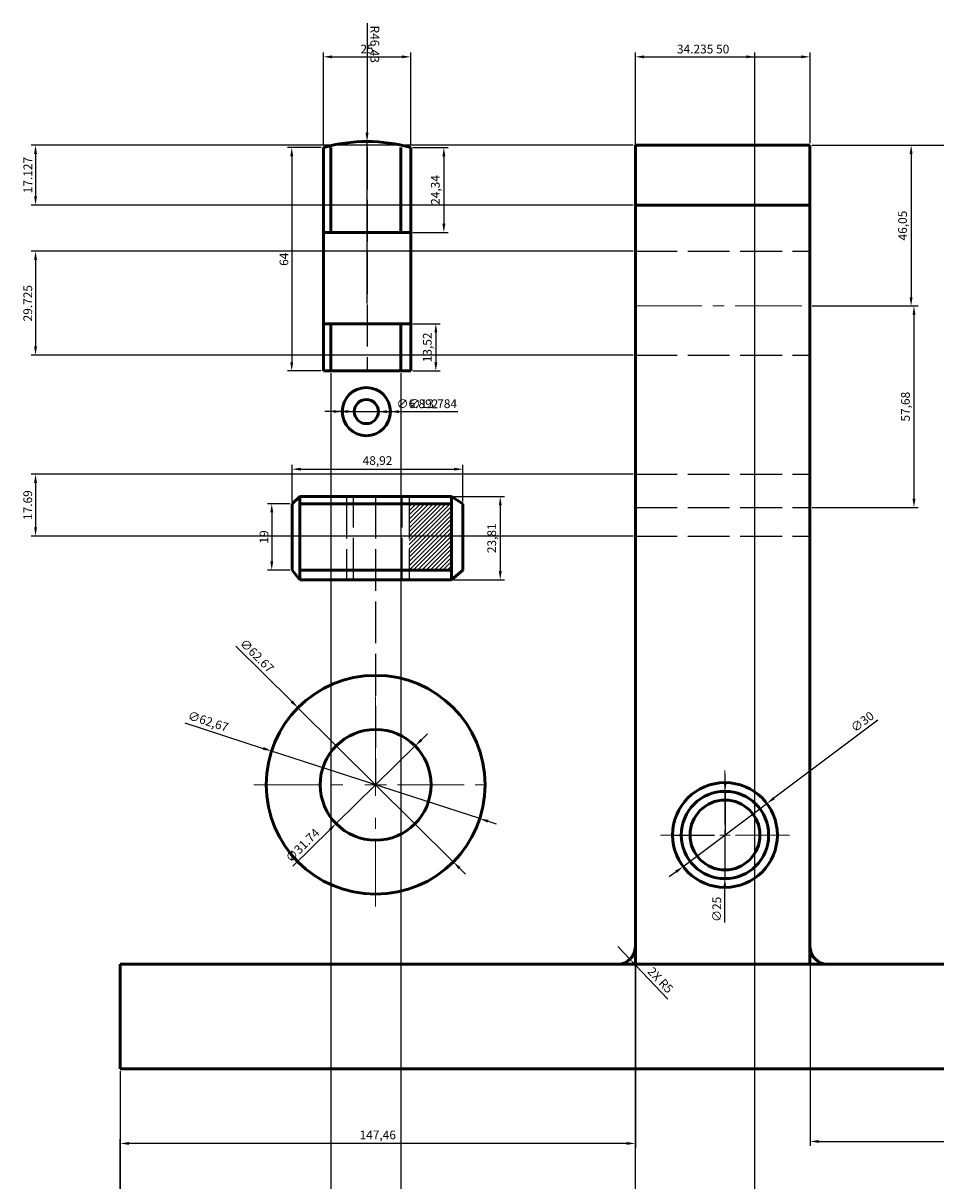
# Model space of a CAD drawing. Units: millimetres. Extents: x 921 to 2648, y 1390 to 2315.
# Tile 2 of 10: x 923 to 1184, y 1882 to 2213. Entities that reach past the tile are written whole.
import ezdxf

# ---------------------------------------------------------------- set-up
doc = ezdxf.new("R2010")
doc.units = ezdxf.units.MM
doc.linetypes.add('ACAD_ISO02W100', pattern=[15, 12, -3])
doc.linetypes.add('CENTER2', pattern=[28.575, 19.05, -3.175, 3.175, -3.175])
for name, color, linetype, lineweight in [('M-CNTR', 1, 'CENTER2', 18), ('M-DIMS', 2, 'Continuous', 25), ('M-HATC', 8, 'Continuous', 18), ('M-HIDN', 4, 'ACAD_ISO02W100', 25), ('M-OUTL', 7, 'Continuous', 50)]:
    doc.layers.add(name, color=color, linetype=linetype, lineweight=lineweight)
doc.styles.get("Standard").update_dxf_attribs({"font": 'arial.ttf'})
doc.dimstyles.new('ISO-25', dxfattribs={"dimtxt": 2.5, "dimasz": 2.5, "dimexe": 1.25, "dimexo": 0.625, "dimtad": 1, "dimtxsty": 'Standard', "dimcen": 2.5, "dimadec": 0, "dimazin": 0, "dimtfac": 1, "dimtmove": 0, "dimatfit": 3, "dimfxl": 1, "dimarcsym": 0})

# ---------------------------------------------------------------- blocks, each defined once
blk = doc.blocks.new('*D1')
at = {"layer": 'Defpoints', "color": 0, "transparency": 16777216}
for p in [(1033.77, 2177.55), (1033.77, 2153.21), (1043.26, 2153.21)]:
    blk.add_point(p, dxfattribs=at)
at = {"layer": 'M-DIMS', "color": 0, "lineweight": -2, "transparency": 16777216}
for p, q in [((1034.4, 2177.55), (1044.51, 2177.55)), ((1043.26, 2175.05), (1043.26, 2155.71)), ((1034.4, 2153.21), (1044.51, 2153.21))]:
    blk.add_line(p, q, dxfattribs=at)
at = {"layer": 'M-DIMS', "color": 0, "transparency": 16777216}
for points in [[(1042.85, 2175.05), (1043.68, 2175.05), (1043.26, 2177.55)], [(1042.85, 2155.71), (1043.68, 2155.71), (1043.26, 2153.21)]]:
    blk.add_solid(points, dxfattribs=at)
at = {"layer": 'M-DIMS', "color": 0, "transparency": 16777216, "insert": (1041.14, 2165.38), "char_height": 2.5, "attachment_point": 5, "rotation": 90}
blk.add_mtext('24,34', dxfattribs=at)
blk = doc.blocks.new('*D2')
at = {"layer": 'Defpoints', "color": 0, "transparency": 16777216}
for p in [(1033.77, 2127.07), (1033.77, 2113.55), (1040.96, 2113.55)]:
    blk.add_point(p, dxfattribs=at)
at = {"layer": 'M-DIMS', "color": 0, "lineweight": -2, "transparency": 16777216}
for p, q in [((1034.4, 2127.07), (1042.21, 2127.07)), ((1040.96, 2124.57), (1040.96, 2116.05)), ((1034.4, 2113.55), (1042.21, 2113.55))]:
    blk.add_line(p, q, dxfattribs=at)
at = {"layer": 'M-DIMS', "color": 0, "transparency": 16777216}
for points in [[(1040.55, 2124.57), (1041.38, 2124.57), (1040.96, 2127.07)], [(1040.55, 2116.05), (1041.38, 2116.05), (1040.96, 2113.55)]]:
    blk.add_solid(points, dxfattribs=at)
at = {"layer": 'M-DIMS', "color": 0, "transparency": 16777216, "insert": (1038.84, 2120.31), "char_height": 2.5, "attachment_point": 5, "rotation": 90}
blk.add_mtext('13,52', dxfattribs=at)
blk = doc.blocks.new('*D3')
at = {"layer": 'Defpoints', "color": 0, "transparency": 16777216}
for p in [(1008.77, 2177.55), (999.71, 2113.55), (1008.77, 2113.55)]:
    blk.add_point(p, dxfattribs=at)
at = {"layer": 'M-DIMS', "color": 0, "lineweight": -2, "transparency": 16777216}
for p, q in [((1008.15, 2177.55), (998.46, 2177.55)), ((999.71, 2175.05), (999.71, 2116.05)), ((1008.15, 2113.55), (998.46, 2113.55))]:
    blk.add_line(p, q, dxfattribs=at)
at = {"layer": 'M-DIMS', "color": 0, "transparency": 16777216}
for points in [[(999.29, 2175.05), (1000.12, 2175.05), (999.71, 2177.55)], [(999.29, 2116.05), (1000.12, 2116.05), (999.71, 2113.55)]]:
    blk.add_solid(points, dxfattribs=at)
at = {"layer": 'M-DIMS', "color": 0, "transparency": 16777216, "insert": (997.8, 2145.55), "char_height": 2.5, "attachment_point": 5, "rotation": 90}
blk.add_mtext('64', dxfattribs=at)
blk = doc.blocks.new('*U4')
at = {"layer": 'M-CNTR', "color": 0, "transparency": 16777216}
for p, q in [((0, 6.27), (0, 34.83)), ((-34.83, 0), (-6.27, 0)), ((6.27, 0), (34.83, 0)), ((0, -34.83), (0, -6.27))]:
    blk.add_line(p, q, dxfattribs=at)
at = {"layer": 'M-CNTR', "color": 0, "linetype": 'Continuous', "transparency": 16777216}
for p, q in [((-3.13, 0), (3.13, 0)), ((0, -3.13), (0, 3.13))]:
    blk.add_line(p, q, dxfattribs=at)
blk = doc.blocks.new('*U5')
at = {"layer": 'M-CNTR', "color": 0, "transparency": 16777216}
for p, q in [((0, 3), (0, 18.5)), ((-18.5, 0), (-3, 0)), ((3, 0), (18.5, 0)), ((0, -18.5), (0, -3))]:
    blk.add_line(p, q, dxfattribs=at)
at = {"layer": 'M-CNTR', "color": 0, "linetype": 'Continuous', "transparency": 16777216}
for p, q in [((-1.5, 0), (1.5, 0)), ((0, -1.5), (0, 1.5))]:
    blk.add_line(p, q, dxfattribs=at)
blk = doc.blocks.new('*D6')
at = {"layer": 'Defpoints', "color": 0, "transparency": 16777216}
for p in [(1048.72, 2085.43), (999.8, 2075.52), (1048.72, 2075.52)]:
    blk.add_point(p, dxfattribs=at)
at = {"layer": 'M-DIMS', "color": 0, "lineweight": -2, "transparency": 16777216}
for p, q in [((999.8, 2076.14), (999.8, 2086.68)), ((1002.3, 2085.43), (1046.22, 2085.43)), ((1048.72, 2076.14), (1048.72, 2086.68))]:
    blk.add_line(p, q, dxfattribs=at)
at = {"layer": 'M-DIMS', "color": 0, "transparency": 16777216}
for points in [[(1002.3, 2085.85), (1002.3, 2085.01), (999.8, 2085.43)], [(1046.22, 2085.85), (1046.22, 2085.01), (1048.72, 2085.43)]]:
    blk.add_solid(points, dxfattribs=at)
at = {"layer": 'M-DIMS', "color": 0, "transparency": 16777216, "insert": (1024.26, 2087.56), "char_height": 2.5, "attachment_point": 5}
blk.add_mtext('48,92', dxfattribs=at)
blk = doc.blocks.new('*D7')
at = {"layer": 'Defpoints', "color": 0, "transparency": 16777216}
for p in [(1045.45, 2077.56), (1045.45, 2053.75), (1059.4, 2053.75)]:
    blk.add_point(p, dxfattribs=at)
at = {"layer": 'M-DIMS', "color": 0, "lineweight": -2, "transparency": 16777216}
for p, q in [((1046.07, 2077.56), (1060.65, 2077.56)), ((1059.4, 2075.06), (1059.4, 2056.25)), ((1046.07, 2053.75), (1060.65, 2053.75))]:
    blk.add_line(p, q, dxfattribs=at)
at = {"layer": 'M-DIMS', "color": 0, "transparency": 16777216}
for points in [[(1058.99, 2075.06), (1059.82, 2075.06), (1059.4, 2077.56)], [(1058.99, 2056.25), (1059.82, 2056.25), (1059.4, 2053.75)]]:
    blk.add_solid(points, dxfattribs=at)
at = {"layer": 'M-DIMS', "color": 0, "transparency": 16777216, "insert": (1057.28, 2065.65), "char_height": 2.5, "attachment_point": 5, "rotation": 90}
blk.add_mtext('23,81', dxfattribs=at)
blk = doc.blocks.new('*D8')
at = {"layer": 'Defpoints', "color": 0, "transparency": 16777216}
for p in [(999.8, 2075.52), (993.99, 2056.52), (999.8, 2056.52)]:
    blk.add_point(p, dxfattribs=at)
at = {"layer": 'M-DIMS', "color": 0, "lineweight": -2, "transparency": 16777216}
for p, q in [((999.18, 2075.52), (992.74, 2075.52)), ((993.99, 2073.02), (993.99, 2059.02)), ((999.18, 2056.52), (992.74, 2056.52))]:
    blk.add_line(p, q, dxfattribs=at)
at = {"layer": 'M-DIMS', "color": 0, "transparency": 16777216}
for points in [[(993.57, 2073.02), (994.41, 2073.02), (993.99, 2075.52)], [(993.57, 2059.02), (994.41, 2059.02), (993.99, 2056.52)]]:
    blk.add_solid(points, dxfattribs=at)
at = {"layer": 'M-DIMS', "color": 0, "transparency": 16777216, "insert": (992.09, 2066.02), "char_height": 2.5, "attachment_point": 5, "rotation": 90}
blk.add_mtext('19', dxfattribs=at)
blk = doc.blocks.new('*D9')
at = {"layer": 'Defpoints', "color": 0, "transparency": 16777216}
for p in [(993.92, 2004.7), (1053.53, 1985.37)]:
    blk.add_point(p, dxfattribs=at)
at = {"layer": 'M-DIMS', "color": 0, "lineweight": -2, "transparency": 16777216}
for p, q in [((969.13, 2012.74), (991.54, 2005.47)), ((1053.53, 1985.37), (993.92, 2004.7)), ((1055.91, 1984.6), (1058.28, 1983.83))]:
    blk.add_line(p, q, dxfattribs=at)
at = {"layer": 'M-DIMS', "color": 0, "transparency": 16777216}
for points in [[(991.67, 2005.87), (991.41, 2005.08), (993.92, 2004.7)], [(1056.03, 1984.99), (1055.78, 1984.2), (1053.53, 1985.37)]]:
    blk.add_solid(points, dxfattribs=at)
at = {"layer": 'M-DIMS', "color": 0, "transparency": 16777216, "insert": (975.7, 2012.89), "char_height": 2.5, "attachment_point": 5, "rotation": 342.0306}
blk.add_mtext('∅62,67', dxfattribs=at)
blk = doc.blocks.new('*D10')
at = {"layer": 'Defpoints', "color": 0, "transparency": 16777216}
for p in [(1148.08, 2178.21), (1148.08, 2132.16), (1177.03, 2132.16)]:
    blk.add_point(p, dxfattribs=at)
at = {"layer": 'M-DIMS', "color": 0, "lineweight": -2, "transparency": 16777216}
for p, q in [((1148.7, 2178.21), (1178.28, 2178.21)), ((1177.03, 2175.71), (1177.03, 2134.66)), ((1148.7, 2132.16), (1178.28, 2132.16))]:
    blk.add_line(p, q, dxfattribs=at)
at = {"layer": 'M-DIMS', "color": 0, "transparency": 16777216}
for points in [[(1176.61, 2175.71), (1177.44, 2175.71), (1177.03, 2178.21)], [(1176.61, 2134.66), (1177.44, 2134.66), (1177.03, 2132.16)]]:
    blk.add_solid(points, dxfattribs=at)
at = {"layer": 'M-DIMS', "color": 0, "transparency": 16777216, "insert": (1174.9, 2155.19), "char_height": 2.5, "attachment_point": 5, "rotation": 90}
blk.add_mtext('46,05', dxfattribs=at)
blk = doc.blocks.new('*D11')
at = {"layer": 'Defpoints', "color": 0, "transparency": 16777216}
for p in [(1148.08, 2132.16), (1148.08, 2074.48), (1177.84, 2074.48)]:
    blk.add_point(p, dxfattribs=at)
at = {"layer": 'M-DIMS', "color": 0, "lineweight": -2, "transparency": 16777216}
for p, q in [((1148.7, 2132.16), (1179.09, 2132.16)), ((1177.84, 2129.66), (1177.84, 2076.98)), ((1148.7, 2074.48), (1179.09, 2074.48))]:
    blk.add_line(p, q, dxfattribs=at)
at = {"layer": 'M-DIMS', "color": 0, "transparency": 16777216}
for points in [[(1177.43, 2129.66), (1178.26, 2129.66), (1177.84, 2132.16)], [(1177.43, 2076.98), (1178.26, 2076.98), (1177.84, 2074.48)]]:
    blk.add_solid(points, dxfattribs=at)
at = {"layer": 'M-DIMS', "color": 0, "transparency": 16777216, "insert": (1175.72, 2103.32), "char_height": 2.5, "attachment_point": 5, "rotation": 90}
blk.add_mtext('57,68', dxfattribs=at)
blk = doc.blocks.new('*D12')
at = {"layer": 'Defpoints', "color": 0, "transparency": 16777216}
for p in [(1135.73, 1989.67), (1111.75, 1971.64)]:
    blk.add_point(p, dxfattribs=at)
at = {"layer": 'M-DIMS', "color": 0, "lineweight": -2, "transparency": 16777216}
for p, q in [((1167.46, 2013.52), (1137.73, 1991.17)), ((1111.75, 1971.64), (1135.73, 1989.67)), ((1109.75, 1970.14), (1107.75, 1968.64))]:
    blk.add_line(p, q, dxfattribs=at)
at = {"layer": 'M-DIMS', "color": 0, "transparency": 16777216}
for points in [[(1137.48, 1991.5), (1137.98, 1990.84), (1135.73, 1989.67)], [(1109.5, 1970.47), (1110, 1969.81), (1111.75, 1971.64)]]:
    blk.add_solid(points, dxfattribs=at)
at = {"layer": 'M-DIMS', "color": 0, "transparency": 16777216, "insert": (1163.26, 2012.83), "char_height": 2.5, "attachment_point": 5, "rotation": 36.9285}
blk.add_mtext('∅30', dxfattribs=at)
blk = doc.blocks.new('*D17')
at = {"layer": 'Defpoints', "color": 0, "transparency": 16777216}
for p in [(1098.08, 1948.7), (950.61, 1892.33), (950.61, 1878.16)]:
    blk.add_point(p, dxfattribs=at)
at = {"layer": 'M-DIMS', "color": 0, "lineweight": -2, "transparency": 16777216}
for p, q in [((1098.08, 1948.07), (1098.08, 1891.08)), ((950.61, 1878.78), (950.61, 1893.58)), ((1095.58, 1892.33), (953.11, 1892.33))]:
    blk.add_line(p, q, dxfattribs=at)
at = {"layer": 'M-DIMS', "color": 0, "transparency": 16777216}
for points in [[(953.11, 1892.74), (953.11, 1891.91), (950.61, 1892.33)], [(1095.58, 1892.74), (1095.58, 1891.91), (1098.08, 1892.33)]]:
    blk.add_solid(points, dxfattribs=at)
at = {"layer": 'M-DIMS', "color": 0, "transparency": 16777216, "insert": (1024.34, 1894.45), "char_height": 2.5, "attachment_point": 5}
blk.add_mtext('147,46', dxfattribs=at)
blk = doc.blocks.new('*D18')
at = {"layer": 'Defpoints', "color": 0, "transparency": 16777216}
for p in [(1148.08, 1948.7), (1294.79, 1892.9), (1294.79, 1878.16)]:
    blk.add_point(p, dxfattribs=at)
at = {"layer": 'M-DIMS', "color": 0, "lineweight": -2, "transparency": 16777216}
for p, q in [((1148.08, 1948.07), (1148.08, 1891.65)), ((1294.79, 1878.78), (1294.79, 1894.15)), ((1150.58, 1892.9), (1292.29, 1892.9))]:
    blk.add_line(p, q, dxfattribs=at)
at = {"layer": 'M-DIMS', "color": 0, "transparency": 16777216}
for points in [[(1150.58, 1893.32), (1150.58, 1892.48), (1148.08, 1892.9)], [(1292.29, 1893.32), (1292.29, 1892.48), (1294.79, 1892.9)]]:
    blk.add_solid(points, dxfattribs=at)
at = {"layer": 'M-DIMS', "color": 0, "transparency": 16777216, "insert": (1221.43, 1895.03), "char_height": 2.5, "attachment_point": 5}
blk.add_mtext('146,72', dxfattribs=at)
blk = doc.blocks.new('*D41')
at = {"layer": 'Defpoints', "color": 0, "transparency": 16777216}
for p in [(1148.08, 2203.51), (1098.08, 2178.21), (1148.08, 2178.21)]:
    blk.add_point(p, dxfattribs=at)
at = {"layer": 'M-DIMS', "color": 0, "lineweight": -2, "transparency": 16777216}
for p, q in [((1098.08, 2178.83), (1098.08, 2204.76)), ((1100.58, 2203.51), (1145.58, 2203.51)), ((1148.08, 2178.83), (1148.08, 2204.76))]:
    blk.add_line(p, q, dxfattribs=at)
at = {"layer": 'M-DIMS', "color": 0, "transparency": 16777216}
for points in [[(1100.58, 2203.93), (1100.58, 2203.1), (1098.08, 2203.51)], [(1145.58, 2203.93), (1145.58, 2203.1), (1148.08, 2203.51)]]:
    blk.add_solid(points, dxfattribs=at)
at = {"layer": 'M-DIMS', "color": 0, "transparency": 16777216, "insert": (1123.08, 2205.42), "char_height": 2.5, "attachment_point": 5}
blk.add_mtext('50', dxfattribs=at)
blk = doc.blocks.new('*D42')
at = {"layer": 'Defpoints', "color": 0, "transparency": 16777216}
for p in [(1098.08, 2178.21), (926.36, 2161.08), (1098.08, 2161.08)]:
    blk.add_point(p, dxfattribs=at)
at = {"layer": 'M-DIMS', "color": 0, "lineweight": -2, "transparency": 16777216}
for p, q in [((1097.45, 2178.21), (925.11, 2178.21)), ((926.36, 2175.71), (926.36, 2163.58)), ((1097.45, 2161.08), (925.11, 2161.08))]:
    blk.add_line(p, q, dxfattribs=at)
at = {"layer": 'M-DIMS', "color": 0, "transparency": 16777216}
for points in [[(925.95, 2175.71), (926.78, 2175.71), (926.36, 2178.21)], [(925.95, 2163.58), (926.78, 2163.58), (926.36, 2161.08)]]:
    blk.add_solid(points, dxfattribs=at)
at = {"layer": 'M-DIMS', "color": 0, "transparency": 16777216, "insert": (924.48, 2169.65), "char_height": 2.5, "attachment_point": 5, "rotation": 90}
blk.add_mtext('17.127', dxfattribs=at)
blk = doc.blocks.new('*D43')
at = {"layer": 'Defpoints', "color": 0, "transparency": 16777216}
for p in [(1098.08, 2147.83), (926.36, 2118.1), (1098.08, 2118.1)]:
    blk.add_point(p, dxfattribs=at)
at = {"layer": 'M-DIMS', "color": 0, "lineweight": -2, "transparency": 16777216}
for p, q in [((1097.45, 2147.83), (925.11, 2147.83)), ((926.36, 2145.33), (926.36, 2120.6)), ((1097.45, 2118.1), (925.11, 2118.1))]:
    blk.add_line(p, q, dxfattribs=at)
at = {"layer": 'M-DIMS', "color": 0, "transparency": 16777216}
for points in [[(925.95, 2145.33), (926.78, 2145.33), (926.36, 2147.83)], [(925.95, 2120.6), (926.78, 2120.6), (926.36, 2118.1)]]:
    blk.add_solid(points, dxfattribs=at)
at = {"layer": 'M-DIMS', "color": 0, "transparency": 16777216, "insert": (924.46, 2132.96), "char_height": 2.5, "attachment_point": 5, "rotation": 90}
blk.add_mtext('29.725', dxfattribs=at)
blk = doc.blocks.new('*D44')
at = {"layer": 'Defpoints', "color": 0, "transparency": 16777216}
for p in [(1098.08, 2083.98), (926.36, 2066.28), (1098.08, 2066.28)]:
    blk.add_point(p, dxfattribs=at)
at = {"layer": 'M-DIMS', "color": 0, "lineweight": -2, "transparency": 16777216}
for p, q in [((1097.45, 2083.98), (925.11, 2083.98)), ((926.36, 2081.48), (926.36, 2068.78)), ((1097.45, 2066.28), (925.11, 2066.28))]:
    blk.add_line(p, q, dxfattribs=at)
at = {"layer": 'M-DIMS', "color": 0, "transparency": 16777216}
for points in [[(925.95, 2081.48), (926.78, 2081.48), (926.36, 2083.98)], [(925.95, 2068.78), (926.78, 2068.78), (926.36, 2066.28)]]:
    blk.add_solid(points, dxfattribs=at)
at = {"layer": 'M-DIMS', "color": 0, "transparency": 16777216, "insert": (924.46, 2075.13), "char_height": 2.5, "attachment_point": 5, "rotation": 90}
blk.add_mtext('17.69', dxfattribs=at)
blk = doc.blocks.new('*D46')
at = {"layer": 'Defpoints', "color": 0, "transparency": 16777216}
for p in [(1148.08, 2178.21), (1294.79, 1913.7), (1319.04, 1913.7)]:
    blk.add_point(p, dxfattribs=at)
at = {"layer": 'M-DIMS', "color": 0, "lineweight": -2, "transparency": 16777216}
for p, q in [((1148.7, 2178.21), (1320.29, 2178.21)), ((1319.04, 2175.71), (1319.04, 1916.2)), ((1295.42, 1913.7), (1320.29, 1913.7))]:
    blk.add_line(p, q, dxfattribs=at)
at = {"layer": 'M-DIMS', "color": 0, "transparency": 16777216}
for points in [[(1318.63, 2175.71), (1319.46, 2175.71), (1319.04, 2178.21)], [(1318.63, 1916.2), (1319.46, 1916.2), (1319.04, 1913.7)]]:
    blk.add_solid(points, dxfattribs=at)
at = {"layer": 'M-DIMS', "color": 0, "transparency": 16777216, "insert": (1317.14, 2045.95), "char_height": 2.5, "attachment_point": 5, "rotation": 90}
blk.add_mtext('264.5', dxfattribs=at)
blk = doc.blocks.new('*D49')
at = {"layer": 'Defpoints', "color": 0, "transparency": 16777216}
for p in [(950.61, 1913.7), (1294.79, 1913.7), (1294.79, 1705.98)]:
    blk.add_point(p, dxfattribs=at)
at = {"layer": 'M-DIMS', "color": 0, "lineweight": -2, "transparency": 16777216}
for p, q in [((950.61, 1913.07), (950.61, 1704.73)), ((1294.79, 1913.07), (1294.79, 1704.73)), ((953.11, 1705.98), (1292.29, 1705.98))]:
    blk.add_line(p, q, dxfattribs=at)
at = {"layer": 'M-DIMS', "color": 0, "transparency": 16777216}
for points in [[(953.11, 1706.4), (953.11, 1705.56), (950.61, 1705.98)], [(1292.29, 1706.4), (1292.29, 1705.56), (1294.79, 1705.98)]]:
    blk.add_solid(points, dxfattribs=at)
at = {"layer": 'M-DIMS', "color": 0, "transparency": 16777216, "insert": (1122.7, 1707.88), "char_height": 2.5, "attachment_point": 5}
blk.add_mtext('344.2', dxfattribs=at)
blk = doc.blocks.new('*D51')
at = {"layer": 'Defpoints', "color": 0, "transparency": 16777216}
for p in [(1132.31, 2203.51), (1098.08, 1817.38), (1132.31, 1818.84)]:
    blk.add_point(p, dxfattribs=at)
at = {"layer": 'M-DIMS', "color": 0, "lineweight": -2, "transparency": 16777216}
for p, q in [((1098.08, 1818), (1098.08, 2204.76)), ((1100.58, 2203.51), (1129.81, 2203.51)), ((1132.31, 1819.47), (1132.31, 2204.76))]:
    blk.add_line(p, q, dxfattribs=at)
at = {"layer": 'M-DIMS', "color": 0, "transparency": 16777216}
for points in [[(1100.58, 2203.93), (1100.58, 2203.1), (1098.08, 2203.51)], [(1129.81, 2203.93), (1129.81, 2203.1), (1132.31, 2203.51)]]:
    blk.add_solid(points, dxfattribs=at)
at = {"layer": 'M-DIMS', "color": 0, "transparency": 16777216, "insert": (1115.19, 2205.42), "char_height": 2.5, "attachment_point": 5}
blk.add_mtext('34.235', dxfattribs=at)
blk = doc.blocks.new('*D52')
at = {"layer": 'Defpoints', "color": 0, "transparency": 16777216}
for p in [(1033.77, 2203.51), (1008.77, 2177.55), (1033.77, 2177.55)]:
    blk.add_point(p, dxfattribs=at)
at = {"layer": 'M-DIMS', "color": 0, "lineweight": -2, "transparency": 16777216}
for p, q in [((1008.77, 2178.18), (1008.77, 2204.76)), ((1011.27, 2203.51), (1031.27, 2203.51)), ((1033.77, 2178.18), (1033.77, 2204.76))]:
    blk.add_line(p, q, dxfattribs=at)
at = {"layer": 'M-DIMS', "color": 0, "transparency": 16777216}
for points in [[(1011.27, 2203.93), (1011.27, 2203.1), (1008.77, 2203.51)], [(1031.27, 2203.93), (1031.27, 2203.1), (1033.77, 2203.51)]]:
    blk.add_solid(points, dxfattribs=at)
at = {"layer": 'M-DIMS', "color": 0, "transparency": 16777216, "insert": (1021.27, 2205.42), "char_height": 2.5, "attachment_point": 5}
blk.add_mtext('25', dxfattribs=at)
blk = doc.blocks.new('*D53')
at = {"layer": 'Defpoints', "color": 0, "transparency": 16777216}
for p in [(1010.93, 2113.55), (1030.91, 2113.55), (1030.91, 1705.98)]:
    blk.add_point(p, dxfattribs=at)
at = {"layer": 'M-DIMS', "color": 0, "lineweight": -2, "transparency": 16777216}
for p, q in [((1010.93, 2112.93), (1010.93, 1704.73)), ((1030.91, 2112.93), (1030.91, 1704.73)), ((1013.43, 1705.98), (1028.41, 1705.98))]:
    blk.add_line(p, q, dxfattribs=at)
at = {"layer": 'M-DIMS', "color": 0, "transparency": 16777216}
for points in [[(1013.43, 1706.4), (1013.43, 1705.56), (1010.93, 1705.98)], [(1028.41, 1706.4), (1028.41, 1705.56), (1030.91, 1705.98)]]:
    blk.add_solid(points, dxfattribs=at)
at = {"layer": 'M-DIMS', "color": 0, "transparency": 16777216, "insert": (1020.92, 1707.88), "char_height": 2.5, "attachment_point": 5}
blk.add_mtext('19.983', dxfattribs=at)
blk = doc.blocks.new('*D121')
at = {"layer": 'Defpoints', "color": 0, "transparency": 16777216}
for p in [(1021.27, 2179.26), (1021.27, 2132.84)]:
    blk.add_point(p, dxfattribs=at)
at = {"layer": 'M-DIMS', "color": 0, "lineweight": -2, "transparency": 16777216}
for p, q in [((1021.27, 2213.16), (1021.27, 2181.76)), ((1021.27, 2132.84), (1021.27, 2179.26))]:
    blk.add_line(p, q, dxfattribs=at)
at = {"layer": 'M-DIMS', "color": 0, "transparency": 16777216}
blk.add_solid([(1021.69, 2181.76), (1020.85, 2181.76), (1021.27, 2179.26)], dxfattribs=at)
at = {"layer": 'M-DIMS', "color": 0, "transparency": 16777216, "insert": (1023.17, 2207.12), "char_height": 2.5, "attachment_point": 5, "rotation": 270.0002}
blk.add_mtext('R46.43', dxfattribs=at)
blk = doc.blocks.new('*D123')
at = {"layer": 'Defpoints', "color": 0, "transparency": 16777216}
for p in [(1001.49, 2017.11), (1045.96, 1972.96)]:
    blk.add_point(p, dxfattribs=at)
at = {"layer": 'M-DIMS', "color": 0, "lineweight": -2, "transparency": 16777216}
for p, q in [((983.75, 2034.73), (999.71, 2018.87)), ((1045.96, 1972.96), (1001.49, 2017.11)), ((1047.73, 1971.19), (1049.5, 1969.43))]:
    blk.add_line(p, q, dxfattribs=at)
at = {"layer": 'M-DIMS', "color": 0, "transparency": 16777216}
for points in [[(1000.01, 2019.17), (999.42, 2018.58), (1001.49, 2017.11)], [(1048.02, 1971.49), (1047.44, 1970.9), (1045.96, 1972.96)]]:
    blk.add_solid(points, dxfattribs=at)
at = {"layer": 'M-DIMS', "color": 0, "transparency": 16777216, "insert": (989.54, 2031.76), "char_height": 2.5, "attachment_point": 5, "rotation": 315.2017}
blk.add_mtext('∅62.67', dxfattribs=at)
blk = doc.blocks.new('*D124')
at = {"layer": 'Defpoints', "color": 0, "transparency": 16777216}
for p in [(1035.04, 2006.16), (1012.41, 1983.91)]:
    blk.add_point(p, dxfattribs=at)
at = {"layer": 'M-DIMS', "color": 0, "lineweight": -2, "transparency": 16777216}
for p, q in [((1036.82, 2007.91), (1038.6, 2009.67)), ((1035.04, 2006.16), (1012.41, 1983.91)), ((1000.01, 1971.71), (1010.63, 1982.15))]:
    blk.add_line(p, q, dxfattribs=at)
at = {"layer": 'M-DIMS', "color": 0, "transparency": 16777216}
for points in [[(1036.53, 2008.21), (1037.11, 2007.62), (1035.04, 2006.16)], [(1010.33, 1982.45), (1010.92, 1981.86), (1012.41, 1983.91)]]:
    blk.add_solid(points, dxfattribs=at)
at = {"layer": 'M-DIMS', "color": 0, "transparency": 16777216, "insert": (1003.04, 1977.46), "char_height": 2.5, "attachment_point": 5, "rotation": 44.525}
blk.add_mtext('∅31.74', dxfattribs=at)
blk = doc.blocks.new('*D126')
at = {"layer": 'Defpoints', "color": 0, "transparency": 16777216}
for p in [(1093.08, 1948.7), (1096.52, 1945.07)]:
    blk.add_point(p, dxfattribs=at)
at = {"layer": 'M-DIMS', "color": 0, "lineweight": -2, "transparency": 16777216}
for p, q in [((1093.08, 1948.7), (1096.52, 1945.07)), ((1107.34, 1933.68), (1098.24, 1943.26))]:
    blk.add_line(p, q, dxfattribs=at)
at = {"layer": 'M-DIMS', "color": 0, "transparency": 16777216}
blk.add_solid([(1098.54, 1943.55), (1097.94, 1942.97), (1096.52, 1945.07)], dxfattribs=at)
at = {"layer": 'M-DIMS', "color": 0, "transparency": 16777216, "insert": (1105.03, 1938.88), "char_height": 2.5, "attachment_point": 5, "rotation": 313.5346}
blk.add_mtext('2X R5', dxfattribs=at)
blk = doc.blocks.new('*D127')
at = {"layer": 'Defpoints', "color": 0, "transparency": 16777216}
for p in [(1123.78, 1993.16), (1123.7, 1968.16)]:
    blk.add_point(p, dxfattribs=at)
at = {"layer": 'M-DIMS', "color": 0, "lineweight": -2, "transparency": 16777216}
for p, q in [((1123.79, 1995.66), (1123.8, 1998.16)), ((1123.78, 1993.16), (1123.7, 1968.16)), ((1123.66, 1955.59), (1123.69, 1965.66))]:
    blk.add_line(p, q, dxfattribs=at)
at = {"layer": 'M-DIMS', "color": 0, "transparency": 16777216}
for points in [[(1123.37, 1995.66), (1124.21, 1995.65), (1123.78, 1993.16)], [(1123.28, 1965.66), (1124.11, 1965.65), (1123.7, 1968.16)]]:
    blk.add_solid(points, dxfattribs=at)
at = {"layer": 'M-DIMS', "color": 0, "transparency": 16777216, "insert": (1121.7, 1959.38), "char_height": 2.5, "attachment_point": 5, "rotation": 89.8137}
blk.add_mtext('∅25', dxfattribs=at)
blk = doc.blocks.new('*D128')
at = {"layer": 'Defpoints', "color": 0, "transparency": 16777216}
for p in [(1014.17, 2101.93), (1027.95, 2101.9)]:
    blk.add_point(p, dxfattribs=at)
at = {"layer": 'M-DIMS', "color": 0, "lineweight": -2, "transparency": 16777216}
for p, q in [((1011.67, 2101.93), (1009.17, 2101.94)), ((1014.17, 2101.93), (1027.95, 2101.9)), ((1047.29, 2101.86), (1030.45, 2101.89))]:
    blk.add_line(p, q, dxfattribs=at)
at = {"layer": 'M-DIMS', "color": 0, "transparency": 16777216}
for points in [[(1011.67, 2102.35), (1011.67, 2101.52), (1014.17, 2101.93)], [(1030.45, 2102.31), (1030.45, 2101.48), (1027.95, 2101.9)]]:
    blk.add_solid(points, dxfattribs=at)
at = {"layer": 'M-DIMS', "color": 0, "transparency": 16777216, "insert": (1040.12, 2103.85), "char_height": 2.5, "attachment_point": 5, "rotation": 359.8848}
blk.add_mtext('∅13.784', dxfattribs=at)
blk = doc.blocks.new('*D129')
at = {"layer": 'Defpoints', "color": 0, "transparency": 16777216}
for p in [(1017.61, 2101.93), (1024.51, 2101.9)]:
    blk.add_point(p, dxfattribs=at)
at = {"layer": 'M-DIMS', "color": 0, "lineweight": -2, "transparency": 16777216}
for p, q in [((1015.11, 2101.94), (1012.61, 2101.95)), ((1017.61, 2101.93), (1024.51, 2101.9)), ((1041.89, 2101.83), (1027.01, 2101.89))]:
    blk.add_line(p, q, dxfattribs=at)
at = {"layer": 'M-DIMS', "color": 0, "transparency": 16777216}
for points in [[(1015.12, 2102.35), (1015.11, 2101.52), (1017.61, 2101.93)], [(1027.01, 2102.31), (1027, 2101.47), (1024.51, 2101.9)]]:
    blk.add_solid(points, dxfattribs=at)
at = {"layer": 'M-DIMS', "color": 0, "transparency": 16777216, "insert": (1035.7, 2103.83), "char_height": 2.5, "attachment_point": 5, "rotation": 359.7775}
blk.add_mtext('∅6.892', dxfattribs=at)

msp = doc.modelspace()

# ---------------------------------------------------------------- hatches: boundary and pattern name
at = {"layer": 'M-HATC'}
h = msp.add_hatch(dxfattribs=at)
h.set_pattern_fill('ANSI31', color=256, scale=0.27)
h.paths.add_polyline_path([(1045.4452, 2075.5156), (1033.3358, 2075.5156), (1033.3358, 2056.5156), (1045.4452, 2056.5156)])

# ---------------------------------------------------------------- linework, layer by layer
at = {"layer": 'M-CNTR'}
msp.add_line((1098.0755, 2132.1608), (1148.0755, 2132.1608), dxfattribs=at)
at = {"layer": 'M-HIDN'}
for p, q in [((1021.2702, 2177.5505), (1021.2702, 2113.5505)), ((1098.0755, 2147.8264), (1148.0755, 2147.8264)), ((1098.0755, 2118.1019), (1148.0755, 2118.1019)), ((1098.0755, 2083.9757), (1148.0755, 2083.9757)), ((1015.4234, 2077.5571), (1015.4234, 2053.7481)), ((1017.4234, 2053.7481), (1017.4234, 2077.5571)), ((1023.7222, 2077.5571), (1023.7222, 1995.0344)), ((1031.3358, 2053.7481), (1031.3358, 2077.5571)), ((1033.3358, 2077.5571), (1033.3358, 2053.7481)), ((1098.0755, 2074.4762), (1148.0755, 2074.4762)), ((1098.0755, 2066.2842), (1148.0755, 2066.2842)), ((1108.7408, 1980.6559), (1123.7408, 1980.6559))]:
    msp.add_line(p, q, dxfattribs=at)
at = {"layer": 'M-OUTL'}
for p, q in [((1008.7702, 2177.5505), (1008.7702, 2113.5505)), ((1010.9275, 2177.5505), (1010.9275, 2153.2139)), ((1030.91, 2153.2139), (1030.91, 2177.5505)), ((1033.7702, 2113.5505), (1033.7702, 2177.5505)), ((1098.0755, 2178.2093), (1098.0755, 1948.699)), ((1098.0755, 2178.2093), (1148.0755, 2178.2093)), ((1148.0755, 1948.699), (1148.0755, 2178.2093)), ((1098.0755, 2161.082), (1148.0755, 2161.082)), ((1008.7702, 2153.2139), (1033.7702, 2153.2139)), ((1008.7702, 2127.0726), (1033.7702, 2127.0726)), ((1010.9275, 2127.0726), (1010.9275, 2113.5505)), ((1030.91, 2113.5505), (1030.91, 2127.0726)), ((1008.7702, 2113.5505), (1033.7702, 2113.5505)), ((999.8032, 2075.5156), (1001.9992, 2077.5571)), ((999.8032, 2075.5156), (999.8032, 2056.5156)), ((1001.9992, 2077.5571), (1045.4452, 2077.5571)), ((1001.9992, 2077.5571), (1001.9992, 2053.7481)), ((1001.9992, 2075.5156), (1045.4452, 2075.5156)), ((1045.4452, 2077.5571), (1045.4452, 2053.7481)), ((1045.4452, 2077.5571), (1048.7232, 2075.5156)), ((1048.7232, 2075.5156), (1048.7232, 2056.5156)), ((999.8032, 2056.5156), (1001.9992, 2053.7481)), ((1045.4452, 2056.5156), (1001.9992, 2056.5156)), ((1045.4452, 2053.7481), (1048.7232, 2056.5156)), ((1045.4452, 2053.7481), (1001.9992, 2053.7481)), ((1098.0755, 1948.699), (1098.0755, 1943.699)), ((1148.0755, 1948.699), (1148.0755, 1943.699)), ((1093.0755, 1943.699), (950.6135, 1943.699)), ((950.6135, 1943.699), (950.6135, 1913.699)), ((1098.0755, 1943.699), (1093.0755, 1943.699)), ((1098.0755, 1943.699), (1148.0755, 1943.699)), ((1148.0755, 1943.699), (1153.0755, 1943.699)), ((1294.7941, 1943.699), (1153.0755, 1943.699)), ((950.6135, 1913.699), (1294.7941, 1913.699))]:
    msp.add_line(p, q, dxfattribs=at)
for centre, radius in [((1021.0594, 2101.9138), 6.892), ((1021.0594, 2101.9138), 3.446), ((1023.7222, 1995.0344), 31.3337), ((1023.7222, 1995.0344), 15.8685), ((1123.7408, 1980.6559), 15), ((1123.7408, 1980.6559), 12.5), ((1123.7408, 1980.6559), 10)]:
    msp.add_circle(centre, radius, dxfattribs=at)
for centre, radius, start, end in [((1021.2702, 2132.8382), 46.4267, 74.38087, 105.61913), ((1093.0755, 1948.699), 5, 270, 0), ((1153.0755, 1948.699), 5, 180, 270)]:
    msp.add_arc(centre, radius, start, end, dxfattribs=at)

# ---------------------------------------------------------------- block references
at = {"layer": 'M-CNTR'}
for name, p in [('*U4', (1023.7222, 1995.0344)), ('*U5', (1123.7408, 1980.6559))]:
    msp.add_blockref(name, p, dxfattribs=at)

# ---------------------------------------------------------------- dimensions: what is measured, and where the dimension line sits
at = {"layer": 'M-DIMS'}
dim = msp.add_radius_dim(center=(1021.2702, 2132.8382), mpoint=(1021.27, 2179.2649), dimstyle='ISO-25', override={"dimdec": 2, "dimlfac": 1, "dimrnd": 0, "dimzin": 0, "dimdsep": 46, "dimlunit": 2}, dxfattribs=at)
dim.commit()
dim.dimension.update_dxf_attribs({"geometry": '*D121', "text_midpoint": (1021.2699, 2207.121), "dimtype": 164})
for base, p1, p2, override, picture, middle in [((1033.7702, 2203.5149), (1008.7702, 2177.5505), (1033.7702, 2177.5505), {"dimdec": 0, "dimlfac": 1, "dimrnd": 0, "dimzin": 0, "dimdsep": 46, "dimlunit": 2}, '*D52', (1021.2702, 2205.4163)), ((1132.3108, 2203.5149), (1098.0755, 1817.3777), (1132.3108, 1818.8422), {"dimdec": 3, "dimlfac": 1, "dimrnd": 0, "dimzin": 0, "dimdsep": 46, "dimlunit": 2}, '*D51', (1115.1932, 2205.4172)), ((1148.0755, 2203.5149), (1098.0755, 2178.2093), (1148.0755, 2178.2093), {"dimdec": 0, "dimlfac": 1, "dimrnd": 0, "dimzin": 0, "dimdsep": 46, "dimlunit": 2}, '*D41', (1123.0755, 2205.4163)), ((1030.90998, 1705.9795), (1010.92747, 2113.5505), (1030.90998, 2113.5505), {"dimdec": 3, "dimlfac": 1, "dimrnd": 0, "dimzin": 0, "dimdsep": 46, "dimlunit": 2}, '*D53', (1020.91873, 1707.88179)), ((1048.7232, 2085.4299), (999.8032, 2075.5156), (1048.7232, 2075.5156), {"dimclrd": 0, "dimclre": 0, "dimclrt": 0}, '*D6', (1024.2632, 2087.5573)), ((950.6135, 1892.3265), (1098.0755, 1948.699), (950.6135, 1878.159), {"dimclrd": 0, "dimclre": 0, "dimclrt": 0}, '*D17', (1024.3445, 1894.4539)), ((1294.7941, 1892.9016), (1148.0755, 1948.699), (1294.7941, 1878.159), {"dimclrd": 0, "dimclre": 0, "dimclrt": 0}, '*D18', (1221.4348, 1895.029)), ((1294.7941, 1705.9795), (950.6135, 1913.699), (1294.7941, 1913.699), {"dimdec": 1, "dimlfac": 1, "dimrnd": 0, "dimzin": 0, "dimdsep": 46, "dimlunit": 2}, '*D49', (1122.7038, 1707.8818))]:
    dim = msp.add_linear_dim(base=base, p1=p1, p2=p2, dimstyle='ISO-25', override=override, dxfattribs=at)
    dim.commit()
    dim.dimension.update_dxf_attribs({"geometry": picture, "text_midpoint": middle})
for base, p1, p2, override, picture, middle in [((926.3635, 2161.082), (1098.0755, 2178.2093), (1098.0755, 2161.082), {"dimdec": 3, "dimlfac": 1, "dimrnd": 0, "dimzin": 0, "dimdsep": 46, "dimlunit": 2}, '*D42', (924.4834, 2169.6456)), ((999.7059, 2113.5505), (1008.7702, 2177.5505), (1008.7702, 2113.5505), {"dimclrd": 0, "dimclre": 0, "dimclrt": 0}, '*D3', (997.8045, 2145.5505)), ((1043.2649, 2153.2139), (1033.7702, 2177.5505), (1033.7702, 2153.2139), {"dimclrd": 0, "dimclre": 0, "dimclrt": 0}, '*D1', (1041.1375, 2165.3822)), ((1177.0251, 2132.1608), (1148.0755, 2178.2093), (1148.0755, 2132.1608), {"dimclrd": 0, "dimclre": 0, "dimclrt": 0}, '*D10', (1174.8978, 2155.185)), ((1319.0441, 1913.699), (1148.0755, 2178.2093), (1294.7941, 1913.699), {"dimdec": 1, "dimlfac": 1, "dimrnd": 0, "dimzin": 0, "dimdsep": 46, "dimlunit": 2}, '*D46', (1317.1427, 2045.9541)), ((926.36349, 2118.1019), (1098.07554, 2147.82644), (1098.07554, 2118.1019), {"dimdec": 3, "dimlfac": 1, "dimrnd": 0, "dimzin": 0, "dimdsep": 46, "dimlunit": 2}, '*D43', (924.46206, 2132.96417)), ((1177.8437, 2074.4762), (1148.0755, 2132.1608), (1148.0755, 2074.4762), {"dimclrd": 0, "dimclre": 0, "dimclrt": 0}, '*D11', (1175.7163, 2103.3185)), ((1040.9648, 2113.5505), (1033.7702, 2127.0726), (1033.7702, 2113.5505), {"dimclrd": 0, "dimclre": 0, "dimclrt": 0}, '*D2', (1038.8374, 2120.3116)), ((926.3635, 2066.2842), (1098.0755, 2083.9757), (1098.0755, 2066.2842), {"dimdec": 2, "dimlfac": 1, "dimrnd": 0, "dimzin": 0, "dimdsep": 46, "dimlunit": 2}, '*D44', (924.4621, 2075.13)), ((993.9888, 2056.5156), (999.8032, 2075.5156), (999.8032, 2056.5156), {"dimclrd": 0, "dimclre": 0, "dimclrt": 0}, '*D8', (992.0874, 2066.0156)), ((1059.4036, 2053.7481), (1045.4452, 2077.5571), (1045.4452, 2053.7481), {"dimclrd": 0, "dimclre": 0, "dimclrt": 0}, '*D7', (1057.2762, 2065.6526))]:
    dim = msp.add_linear_dim(base=base, p1=p1, p2=p2, angle=90, dimstyle='ISO-25', override=override, dxfattribs=at)
    dim.commit()
    dim.dimension.update_dxf_attribs({"geometry": picture, "text_midpoint": middle})
for p1, p2, override, picture, middle in [((1014.1675, 2101.9276), (1027.9514, 2101.8999), {"dimdec": 3, "dimlfac": 1, "dimrnd": 0, "dimzin": 0, "dimdsep": 46, "dimlunit": 2}, '*D128', (1040.1206, 2101.8754)), ((1017.6135, 2101.9271), (1024.5054, 2101.9004), {"dimdec": 3, "dimlfac": 1, "dimrnd": 0, "dimzin": 0, "dimdsep": 46, "dimlunit": 2}, '*D129', (1035.6956, 2101.8569)), ((1123.7815, 1993.1558), (1123.7002, 1968.156), {"dimdec": 0, "dimlfac": 1, "dimrnd": 0, "dimzin": 0, "dimdsep": 46, "dimlunit": 2}, '*D127', (1123.6716, 1959.371))]:
    dim = msp.add_diameter_dim_2p(p1=p1, p2=p2, dimstyle='ISO-25', override=override, dxfattribs=at)
    dim.commit()
    dim.dimension.update_dxf_attribs({"geometry": picture, "text_midpoint": middle})
for p1, p2, override, picture, middle in [((1045.9563, 1972.9562), (1001.4881, 2017.1125), {"dimdec": 2, "dimlfac": 1, "dimrnd": 0, "dimzin": 0, "dimdsep": 46, "dimlunit": 2}, '*D123', (988.1477, 2030.3594)), ((1053.5275, 1985.3677), (993.917, 2004.7011), {"dimclrd": 0, "dimclre": 0, "dimclrt": 0}, '*D9', (975.0351, 2010.825)), ((1111.75, 1971.6436), (1135.7316, 1989.6682), {"dimclrd": 0, "dimclre": 0, "dimclrt": 0}, '*D12', (1164.4471, 2011.2507)), ((1035.0356, 2006.1617), (1012.4089, 1983.9071), {"dimdec": 2, "dimlfac": 1, "dimrnd": 0, "dimzin": 0, "dimdsep": 46, "dimlunit": 2}, '*D124', (1004.4253, 1976.0548))]:
    dim = msp.add_diameter_dim_2p(p1=p1, p2=p2, dimstyle='ISO-25', override=override, dxfattribs=at)
    dim.commit()
    dim.dimension.update_dxf_attribs({"geometry": picture, "text_midpoint": middle, "dimtype": 163})
dim = msp.add_radius_dim(center=(1093.0755, 1948.699), mpoint=(1096.5195, 1945.0742), text='2X <>', dimstyle='ISO-25', override={"dimdec": 0, "dimlfac": 1, "dimrnd": 0, "dimzin": 0, "dimdsep": 46, "dimlunit": 2}, dxfattribs=at)
dim.commit()
dim.dimension.update_dxf_attribs({"geometry": '*D126', "text_midpoint": (1105.032, 1938.8753)})

doc.saveas('drawing.dxf')
